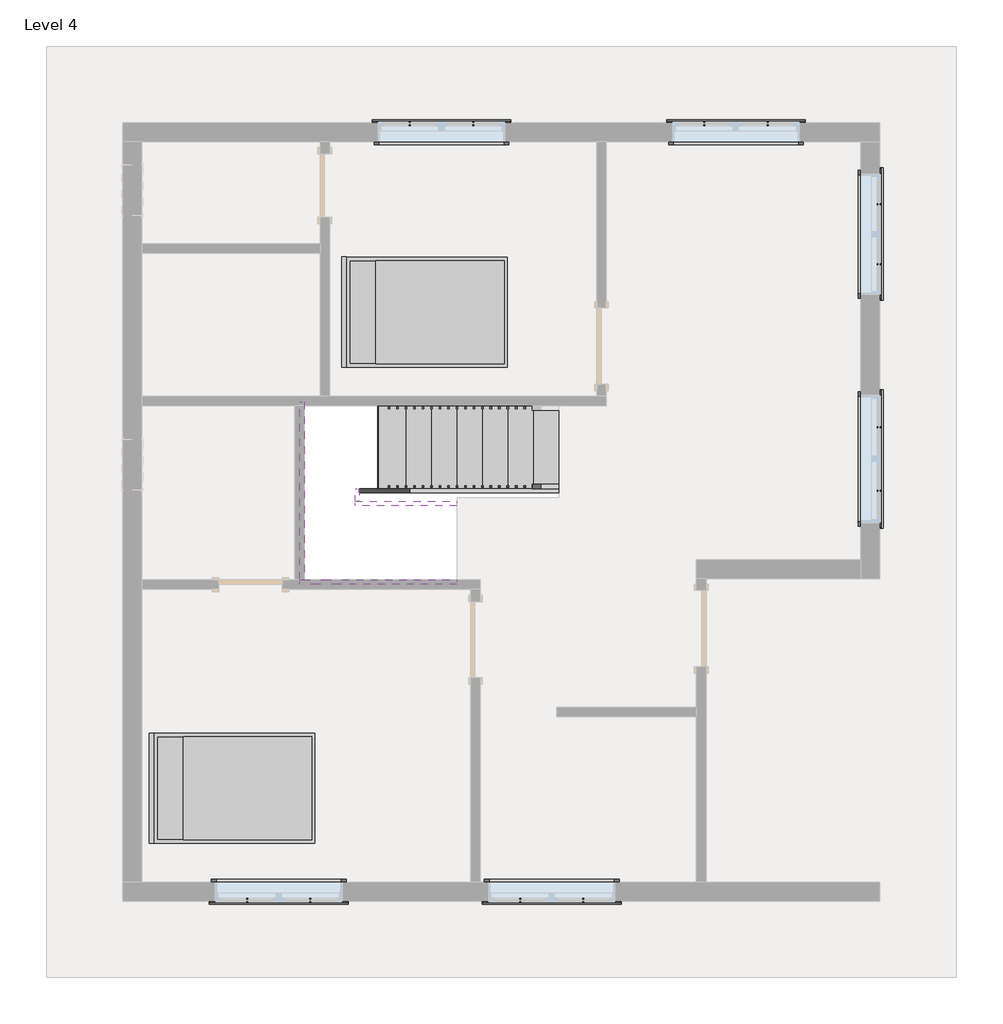
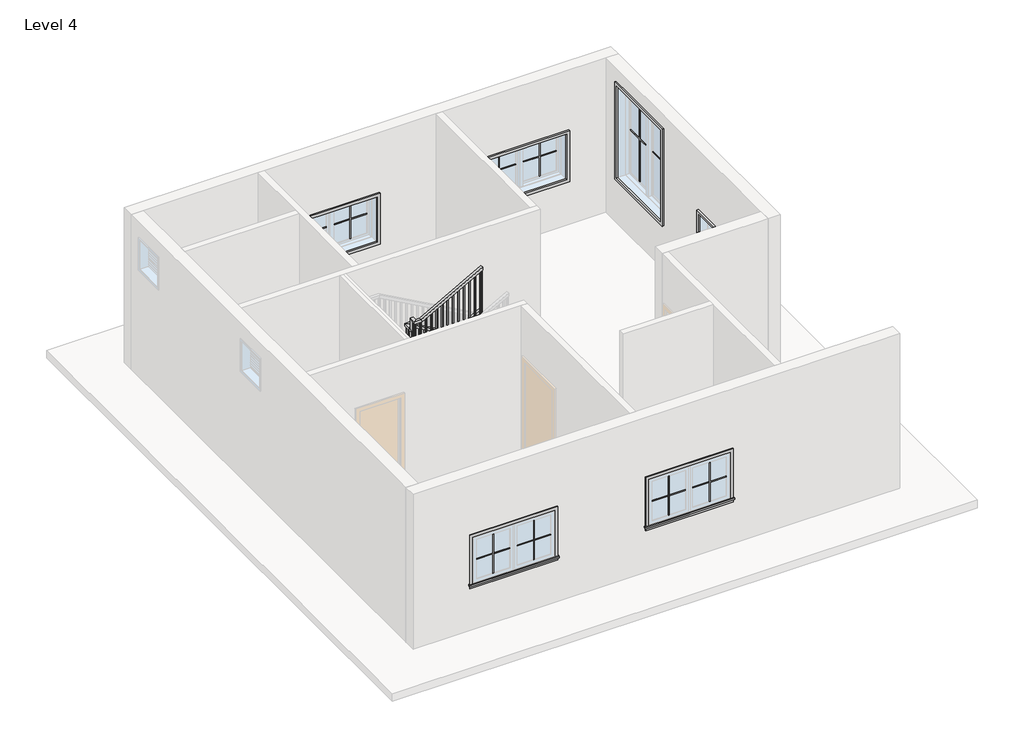
# One storey, part 2 of 2: 24 proxies, 6 members, 2 furniture elements, 1 railing, 1 stair flight.
"""IFC4 building model written with IfcOpenShell, lengths in millimetres."""

from ifc_helpers import new_model, si_unit, frame, origin, place, context, project, spatial, polyline, outline, extrude, faceted_brep, transform, mapped, element, save
from components import muntin_pattern_2x2_muntin_pattern_2x2_9352d081, muntin_pattern_2x2_muntin_pattern_2x2_5c2cbe28, muntin_pattern_2x2_muntin_pattern_2x2_bff912c5, muntin_pattern_2x2_muntin_pattern_2x2_c2194282, trim_window_exterior_flat_with_sill_979bde60, trim_window_exterior_flat_with_sill_e04b3088, trim_window_interior_flat_picture_frame_7883d11b, trim_window_interior_flat_picture_frame_2a7685fe, bed_17739_bed_17739_15c61121, stair_flight_db34188c

model = new_model("IFC4")

# Units and contexts
model_context = context("Model", 3, world=origin())
ifc_project = project(units=[si_unit("LENGTHUNIT", "METRE", prefix="MILLI")], contexts=[model_context])

# Site, building, storey
site = spatial("IfcSite", under=ifc_project)
building = spatial("IfcBuilding", under=site)
storey = spatial("IfcBuildingStorey", under=building, Name="Level 4", Elevation=9448.8)

# Proxies
placement = place(None, origin())
muntin_pattern_2x2_muntin_pattern_2x2_shape = muntin_pattern_2x2_muntin_pattern_2x2_9352d081(model_context)
element("IfcBuildingElementProxy", 1, Name="Muntin Pattern_2x2 : Muntin Pattern_2x2", ObjectType="Muntin Pattern_2x2 : Muntin Pattern_2x2", at=placement, inside=storey, context=model_context, shape_type="MappedRepresentation", body=[
    mapped(muntin_pattern_2x2_muntin_pattern_2x2_shape, transform((-3542.9505704, -5264.0292021, 10433.05), x_axis=(-1.0, 0.0, 0.0), y_axis=(0.0, -1.0, 0.0), z_axis=(0.0, 0.0, 1.0))),
])
element("IfcBuildingElementProxy", 2, Name="Muntin Pattern_2x2 : Muntin Pattern_2x2", ObjectType="Muntin Pattern_2x2 : Muntin Pattern_2x2", at=placement, inside=storey, context=model_context, shape_type="MappedRepresentation", body=[
    mapped(muntin_pattern_2x2_muntin_pattern_2x2_shape, transform((-272.7005704, -5264.0292021, 10433.05), x_axis=(-1.0, 0.0, 0.0), y_axis=(0.0, -1.0, 0.0), z_axis=(0.0, 0.0, 1.0))),
])
element("IfcBuildingElementProxy", 3, Name="Muntin Pattern_2x2 : Muntin Pattern_2x2", ObjectType="Muntin Pattern_2x2 : Muntin Pattern_2x2", at=placement, inside=storey, context=model_context, shape_type="MappedRepresentation", body=[
    mapped(muntin_pattern_2x2_muntin_pattern_2x2_shape, transform((3269.0119296, 401.7582979, 10433.05), x_axis=(0.0, -1.0, 0.0), y_axis=(1.0, 0.0, 0.0), z_axis=(0.0, 0.0, 1.0))),
])
element("IfcBuildingElementProxy", 4, Name="Muntin Pattern_2x2 : Muntin Pattern_2x2", ObjectType="Muntin Pattern_2x2 : Muntin Pattern_2x2", at=placement, inside=storey, context=model_context, shape_type="MappedRepresentation", body=[
    mapped(muntin_pattern_2x2_muntin_pattern_2x2_shape, transform((1175.0994296, 4038.7207979, 10433.05), x_axis=(1.0, 0.0, 0.0), y_axis=(0.0, 1.0, 0.0), z_axis=(0.0, 0.0, 1.0))),
])
element("IfcBuildingElementProxy", 5, Name="Muntin Pattern_2x2 : Muntin Pattern_2x2", ObjectType="Muntin Pattern_2x2 : Muntin Pattern_2x2", at=placement, inside=storey, context=model_context, shape_type="MappedRepresentation", body=[
    mapped(muntin_pattern_2x2_muntin_pattern_2x2_shape, transform((-2352.3255704, 4038.7207979, 10433.05), x_axis=(1.0, 0.0, 0.0), y_axis=(0.0, 1.0, 0.0), z_axis=(0.0, 0.0, 1.0))),
])
muntin_pattern_2x2_muntin_pattern_2x2_2_shape = muntin_pattern_2x2_muntin_pattern_2x2_5c2cbe28(model_context)
element("IfcBuildingElementProxy", 6, Name="Muntin Pattern_2x2 : Muntin Pattern_2x2", ObjectType="Muntin Pattern_2x2 : Muntin Pattern_2x2", at=placement, inside=storey, context=model_context, shape_type="MappedRepresentation", body=[
    mapped(muntin_pattern_2x2_muntin_pattern_2x2_2_shape, transform((-4301.7755704, -5264.0292021, 10433.05), x_axis=(1.0, 0.0, 0.0), y_axis=(0.0, 1.0, 0.0), z_axis=(0.0, 0.0, 1.0))),
])
element("IfcBuildingElementProxy", 7, Name="Muntin Pattern_2x2 : Muntin Pattern_2x2", ObjectType="Muntin Pattern_2x2 : Muntin Pattern_2x2", at=placement, inside=storey, context=model_context, shape_type="MappedRepresentation", body=[
    mapped(muntin_pattern_2x2_muntin_pattern_2x2_2_shape, transform((-1031.5255704, -5264.0292021, 10433.05), x_axis=(1.0, 0.0, 0.0), y_axis=(0.0, 1.0, 0.0), z_axis=(0.0, 0.0, 1.0))),
])
element("IfcBuildingElementProxy", 8, Name="Muntin Pattern_2x2 : Muntin Pattern_2x2", ObjectType="Muntin Pattern_2x2 : Muntin Pattern_2x2", at=placement, inside=storey, context=model_context, shape_type="MappedRepresentation", body=[
    mapped(muntin_pattern_2x2_muntin_pattern_2x2_2_shape, transform((3269.0119296, -357.0667021, 10433.05), x_axis=(0.0, 1.0, 0.0), y_axis=(-1.0, 0.0, 0.0), z_axis=(0.0, 0.0, 1.0))),
])
element("IfcBuildingElementProxy", 9, Name="Muntin Pattern_2x2 : Muntin Pattern_2x2", ObjectType="Muntin Pattern_2x2 : Muntin Pattern_2x2", at=placement, inside=storey, context=model_context, shape_type="MappedRepresentation", body=[
    mapped(muntin_pattern_2x2_muntin_pattern_2x2_2_shape, transform((1933.9244296, 4038.7207979, 10433.05), x_axis=(-1.0, 0.0, 0.0), y_axis=(0.0, -1.0, 0.0), z_axis=(0.0, 0.0, 1.0))),
])
element("IfcBuildingElementProxy", 10, Name="Muntin Pattern_2x2 : Muntin Pattern_2x2", ObjectType="Muntin Pattern_2x2 : Muntin Pattern_2x2", at=placement, inside=storey, context=model_context, shape_type="MappedRepresentation", body=[
    mapped(muntin_pattern_2x2_muntin_pattern_2x2_2_shape, transform((-1593.5005704, 4038.7207979, 10433.05), x_axis=(-1.0, 0.0, 0.0), y_axis=(0.0, -1.0, 0.0), z_axis=(0.0, 0.0, 1.0))),
])
muntin_pattern_2x2_muntin_pattern_2x2_3_shape = muntin_pattern_2x2_muntin_pattern_2x2_bff912c5(model_context)
element("IfcBuildingElementProxy", 11, Name="Muntin Pattern_2x2 : Muntin Pattern_2x2", ObjectType="Muntin Pattern_2x2 : Muntin Pattern_2x2", at=placement, inside=storey, context=model_context, shape_type="MappedRepresentation", body=[
    mapped(muntin_pattern_2x2_muntin_pattern_2x2_3_shape, transform((3269.0119296, 3075.1082979, 10433.05), x_axis=(0.0, -1.0, 0.0), y_axis=(1.0, 0.0, 0.0), z_axis=(0.0, 0.0, 1.0))),
])
muntin_pattern_2x2_muntin_pattern_2x2_4_shape = muntin_pattern_2x2_muntin_pattern_2x2_c2194282(model_context)
element("IfcBuildingElementProxy", 12, Name="Muntin Pattern_2x2 : Muntin Pattern_2x2", ObjectType="Muntin Pattern_2x2 : Muntin Pattern_2x2", at=placement, inside=storey, context=model_context, shape_type="MappedRepresentation", body=[
    mapped(muntin_pattern_2x2_muntin_pattern_2x2_4_shape, transform((3269.0119296, 2354.3832979, 10433.05), x_axis=(0.0, 1.0, 0.0), y_axis=(-1.0, 0.0, 0.0), z_axis=(0.0, 0.0, 1.0))),
])
trim_window_exterior_flat_with_sill_shape = trim_window_exterior_flat_with_sill_979bde60(model_context)
element("IfcBuildingElementProxy", 13, Name="Trim-Window-Exterior-Flat : with Sill", ObjectType="Trim-Window-Exterior-Flat : with Sill", at=placement, inside=storey, context=model_context, shape_type="MappedRepresentation", body=[
    mapped(trim_window_exterior_flat_with_sill_shape, transform((-3922.3630704, -5273.5542021, 11277.6), x_axis=(1.0, 0.0, 0.0), y_axis=(0.0, 0.0, 1.0), z_axis=(0.0, -1.0, 0.0))),
])
element("IfcBuildingElementProxy", 14, Name="Trim-Window-Exterior-Flat : with Sill", ObjectType="Trim-Window-Exterior-Flat : with Sill", at=placement, inside=storey, context=model_context, shape_type="MappedRepresentation", body=[
    mapped(trim_window_exterior_flat_with_sill_shape, transform((-652.1130704, -5273.5542021, 11277.6), x_axis=(1.0, 0.0, 0.0), y_axis=(0.0, 0.0, 1.0), z_axis=(0.0, -1.0, 0.0))),
])
element("IfcBuildingElementProxy", 15, Name="Trim-Window-Exterior-Flat : with Sill", ObjectType="Trim-Window-Exterior-Flat : with Sill", at=placement, inside=storey, context=model_context, shape_type="MappedRepresentation", body=[
    mapped(trim_window_exterior_flat_with_sill_shape, transform((3278.5369296, 22.3457979, 11277.6), x_axis=(0.0, 1.0, 0.0), y_axis=(0.0, 0.0, 1.0), z_axis=(1.0, 0.0, 0.0))),
])
element("IfcBuildingElementProxy", 16, Name="Trim-Window-Exterior-Flat : with Sill", ObjectType="Trim-Window-Exterior-Flat : with Sill", at=placement, inside=storey, context=model_context, shape_type="MappedRepresentation", body=[
    mapped(trim_window_exterior_flat_with_sill_shape, transform((1554.5119296, 4048.2457979, 11277.6), x_axis=(-1.0, 0.0, 0.0), y_axis=(0.0, 0.0, 1.0), z_axis=(0.0, 1.0, 0.0))),
])
element("IfcBuildingElementProxy", 17, Name="Trim-Window-Exterior-Flat : with Sill", ObjectType="Trim-Window-Exterior-Flat : with Sill", at=placement, inside=storey, context=model_context, shape_type="MappedRepresentation", body=[
    mapped(trim_window_exterior_flat_with_sill_shape, transform((-1972.9130704, 4048.2457979, 11277.6), x_axis=(-1.0, 0.0, 0.0), y_axis=(0.0, 0.0, 1.0), z_axis=(0.0, 1.0, 0.0))),
])
trim_window_exterior_flat_with_sill_2_shape = trim_window_exterior_flat_with_sill_e04b3088(model_context)
element("IfcBuildingElementProxy", 18, Name="Trim-Window-Exterior-Flat : with Sill", ObjectType="Trim-Window-Exterior-Flat : with Sill", at=placement, inside=storey, context=model_context, shape_type="MappedRepresentation", body=[
    mapped(trim_window_exterior_flat_with_sill_2_shape, transform((3278.5369296, 2714.7457979, 12192.0), x_axis=(0.0, 1.0, 0.0), y_axis=(0.0, 0.0, 1.0), z_axis=(1.0, 0.0, 0.0))),
])
trim_window_interior_flat_picture_frame_shape = trim_window_interior_flat_picture_frame_7883d11b(model_context)
element("IfcBuildingElementProxy", 19, Name="Trim-Window-Interior-Flat : Picture Frame", ObjectType="Trim-Window-Interior-Flat : Picture Frame", at=placement, inside=storey, context=model_context, shape_type="MappedRepresentation", body=[
    mapped(trim_window_interior_flat_picture_frame_shape, transform((-3922.3630704, -5044.9542021, 11277.6), x_axis=(-1.0, 0.0, 0.0), y_axis=(0.0, 0.0, 1.0), z_axis=(0.0, 1.0, 0.0))),
])
element("IfcBuildingElementProxy", 20, Name="Trim-Window-Interior-Flat : Picture Frame", ObjectType="Trim-Window-Interior-Flat : Picture Frame", at=placement, inside=storey, context=model_context, shape_type="MappedRepresentation", body=[
    mapped(trim_window_interior_flat_picture_frame_shape, transform((-652.1130704, -5044.9542021, 11277.6), x_axis=(-1.0, 0.0, 0.0), y_axis=(0.0, 0.0, 1.0), z_axis=(0.0, 1.0, 0.0))),
])
element("IfcBuildingElementProxy", 21, Name="Trim-Window-Interior-Flat : Picture Frame", ObjectType="Trim-Window-Interior-Flat : Picture Frame", at=placement, inside=storey, context=model_context, shape_type="MappedRepresentation", body=[
    mapped(trim_window_interior_flat_picture_frame_shape, transform((3049.9369296, 22.3457979, 11277.6), x_axis=(0.0, -1.0, 0.0), y_axis=(0.0, 0.0, 1.0), z_axis=(-1.0, 0.0, 0.0))),
])
element("IfcBuildingElementProxy", 22, Name="Trim-Window-Interior-Flat : Picture Frame", ObjectType="Trim-Window-Interior-Flat : Picture Frame", at=placement, inside=storey, context=model_context, shape_type="MappedRepresentation", body=[
    mapped(trim_window_interior_flat_picture_frame_shape, transform((1554.5119296, 3819.6457979, 11277.6), x_axis=(1.0, 0.0, 0.0), y_axis=(0.0, 0.0, 1.0), z_axis=(0.0, -1.0, 0.0))),
])
element("IfcBuildingElementProxy", 23, Name="Trim-Window-Interior-Flat : Picture Frame", ObjectType="Trim-Window-Interior-Flat : Picture Frame", at=placement, inside=storey, context=model_context, shape_type="MappedRepresentation", body=[
    mapped(trim_window_interior_flat_picture_frame_shape, transform((-1972.9130704, 3819.6457979, 11277.6), x_axis=(1.0, 0.0, 0.0), y_axis=(0.0, 0.0, 1.0), z_axis=(0.0, -1.0, 0.0))),
])
trim_window_interior_flat_picture_frame_2_shape = trim_window_interior_flat_picture_frame_2a7685fe(model_context)
element("IfcBuildingElementProxy", 24, Name="Trim-Window-Interior-Flat : Picture Frame", ObjectType="Trim-Window-Interior-Flat : Picture Frame", at=placement, inside=storey, context=model_context, shape_type="MappedRepresentation", body=[
    mapped(trim_window_interior_flat_picture_frame_2_shape, transform((3049.9369296, 2714.7457979, 12192.0), x_axis=(0.0, -1.0, 0.0), y_axis=(0.0, 0.0, 1.0), z_axis=(-1.0, 0.0, 0.0))),
])

# Furniture
bed_17739_bed_17739_shape = bed_17739_bed_17739_15c61121(model_context)
element("IfcFurniture", 25, ObjectType="Bed_17739 : Bed_17739", at=placement, inside=storey, context=model_context, shape_type="MappedRepresentation", body=[
    mapped(bed_17739_bed_17739_shape, transform((-4455.7630704, -3920.5467683, 9448.8), x_axis=(0.0, 1.0, 0.0), y_axis=(-1.0, 0.0, 0.0), z_axis=(0.0, 0.0, 1.0))),
])
element("IfcFurniture", 26, ObjectType="Bed_17739 : Bed_17739", at=placement, inside=storey, context=model_context, shape_type="MappedRepresentation", body=[
    mapped(bed_17739_bed_17739_shape, transform((-2150.7130704, 1781.2957979, 9448.8), x_axis=(0.0, 1.0, 0.0), y_axis=(-1.0, 0.0, 0.0), z_axis=(0.0, 0.0, 1.0))),
])

# Members
element("IfcMember", 27, ObjectType="Stringer - 2\" Width", at=placement, inside=storey, context=model_context, shape_type="SweptSolid", body=[
    extrude(outline(polyline([(9448.8, -569.5630704), (9656.3983948, -569.5630704), (10982.8428392, -2957.1630704), (10634.1641651, -2957.1630704), (9448.8, -823.5075732), (9448.8, -569.5630704)])), frame((0.0, -384.0542021, 0.0), z_axis=(0.0, 1.0, 0.0), x_axis=(0.0, 0.0, 1.0)), (0.0, 0.0, 1.0), 50.8),
])
element("IfcMember", 28, ObjectType="Stringer - 2\" Width", at=placement, inside=storey, context=model_context, shape_type="SweptSolid", body=[
    extrude(outline(polyline([(-3007.9630704, -333.2542021), (-2957.1630704, -333.2542021), (-2957.1630704, -485.6542021), (-3007.9630704, -485.6542021), (-3007.9630704, -333.2542021)])), frame((0.0, 0.0, 10744.2), z_axis=(0.0, 0.0, 1.0), x_axis=(1.0, 0.0, 0.0)), (0.0, 0.0, 1.0), 304.8),
])
element("IfcMember", 29, ObjectType="Stringer - 2\" Width", at=placement, inside=storey, context=model_context, shape_type="SweptSolid", body=[
    extrude(outline(polyline([(11180.3983948, -3007.9630704), (10831.7197207, -3007.9630704), (11509.053054, -1788.7630704), (11857.7317281, -1788.7630704), (11180.3983948, -3007.9630704)])), frame((0.0, -536.4542021, 0.0), z_axis=(0.0, 1.0, 0.0), x_axis=(0.0, 0.0, 1.0)), (0.0, 0.0, 1.0), 50.8),
])
element("IfcMember", 30, ObjectType="Stringer - 2\" Width", at=placement, inside=storey, context=model_context, shape_type="SweptSolid", body=[
    extrude(outline(polyline([(9448.8, -569.5630704), (9656.3983948, -569.5630704), (11049.0, -3076.2459598), (11049.0, -3617.5630704), (11001.053054, -3617.5630704), (9448.8, -823.5075732), (9448.8, -569.5630704)])), frame((0.0, 657.3457979, 0.0), z_axis=(0.0, 1.0, 0.0), x_axis=(0.0, 0.0, 1.0)), (0.0, 0.0, 1.0), 50.8),
])
element("IfcMember", 31, ObjectType="Stringer - 2\" Width", at=placement, inside=storey, context=model_context, shape_type="SweptSolid", body=[
    extrude(outline(polyline([(-3668.3630704, 708.1457979), (-3617.5630704, 708.1457979), (-3617.5630704, -1425.4542021), (-3668.3630704, -1425.4542021), (-3668.3630704, 708.1457979)])), frame((0.0, 0.0, 10744.2), z_axis=(0.0, 0.0, 1.0), x_axis=(1.0, 0.0, 0.0)), (0.0, 0.0, 1.0), 304.8),
])
element("IfcMember", 32, ObjectType="Stringer - 2\" Width", at=placement, inside=storey, context=model_context, shape_type="SweptSolid", body=[
    extrude(outline(polyline([(10813.5095059, -3668.3630704), (10744.2, -3668.3630704), (10744.2, -3165.4985677), (11509.053054, -1788.7630704), (11857.7317281, -1788.7630704), (10813.5095059, -3668.3630704)])), frame((0.0, -1476.2542021, 0.0), z_axis=(0.0, 1.0, 0.0), x_axis=(0.0, 0.0, 1.0)), (0.0, 0.0, 1.0), 50.8),
])

# Railing
element("IfcRailing", 33, ObjectType="Handrail - Rectangular", at=placement, inside=storey, context=model_context, shape_type="SolidModel", body=[
    faceted_brep([(-569.5630704, -333.2542021, 10532.5333333), (-569.5630704, -333.2542021, 10474.420221), (-569.5630704, -282.4542021, 10474.420221), (-569.5630704, -282.4542021, 10532.5333333), (-2931.7630704, -333.2542021, 11844.8666667), (-2982.5630704, -333.2542021, 11814.9757765), (-2982.5630704, -282.4542021, 11814.9757765), (-2931.7630704, -282.4542021, 11844.8666667), (-2931.7630704, -333.2542021, 11887.2), (-2982.5630704, -333.2542021, 11836.4), (-2982.5630704, -282.4542021, 11836.4), (-2931.7630704, -282.4542021, 11887.2), (-3007.9630704, -333.2542021, 11887.2), (-3007.9630704, -333.2542021, 11836.4), (-3058.7630704, -282.4542021, 11836.4), (-3058.7630704, -282.4542021, 11887.2), (-3007.9630704, -409.4542021, 11887.2), (-3007.9630704, -409.4542021, 11836.4), (-3058.7630704, -409.4542021, 11836.4), (-3058.7630704, -409.4542021, 11887.2), (-3007.9630704, -460.2542021, 11887.2), (-3007.9630704, -511.0542021, 11836.4), (-3058.7630704, -511.0542021, 11836.4), (-3058.7630704, -460.2542021, 11887.2), (-3007.9630704, -460.2542021, 12098.8666667), (-3007.9630704, -511.0542021, 12048.0666667), (-3058.7630704, -511.0542021, 12048.0666667), (-3058.7630704, -460.2542021, 12098.8666667), (-3007.9630704, -536.4542021, 12098.8666667), (-3007.9630704, -536.4542021, 12048.0666667), (-3058.7630704, -587.2542021, 12048.0666667), (-3058.7630704, -587.2542021, 12098.8666667), (-2931.7630704, -536.4542021, 12098.8666667), (-2918.5994682, -536.4542021, 12048.0666667), (-2918.5994682, -587.2542021, 12048.0666667), (-2931.7630704, -587.2542021, 12098.8666667), (-1788.7630704, -536.4542021, 12733.8666667), (-1788.7630704, -587.2542021, 12733.8666667), (-1788.7630704, -587.2542021, 12675.7535543), (-1788.7630704, -536.4542021, 12675.7535543)], [[[0, 1, 2, 3]], [[1, 0, 4, 5]], [[2, 1, 5, 6]], [[3, 2, 6, 7]], [[0, 3, 7, 4]], [[5, 4, 8, 9]], [[6, 5, 9, 10]], [[7, 6, 10, 11]], [[4, 7, 11, 8]], [[9, 8, 12, 13]], [[10, 9, 13, 14]], [[11, 10, 14, 15]], [[8, 11, 15, 12]], [[13, 12, 16, 17]], [[14, 13, 17, 18]], [[15, 14, 18, 19]], [[12, 15, 19, 16]], [[17, 16, 20, 21]], [[18, 17, 21, 22]], [[19, 18, 22, 23]], [[16, 19, 23, 20]], [[21, 20, 24, 25]], [[22, 21, 25, 26]], [[23, 22, 26, 27]], [[20, 23, 27, 24]], [[25, 24, 28, 29]], [[26, 25, 29, 30]], [[27, 26, 30, 31]], [[24, 27, 31, 28]], [[29, 28, 32, 33]], [[30, 29, 33, 34]], [[31, 30, 34, 35]], [[28, 31, 35, 32]], [[36, 37, 38, 39]], [[33, 32, 36, 39]], [[34, 33, 39, 38]], [[35, 34, 38, 37]], [[32, 35, 37, 36]]]),
    extrude(outline(polyline([(12656.3507765, -1823.6880704), (11650.1333333, -1823.6880704), (11650.1333333, -1804.6380704), (12666.9341099, -1804.6380704), (12656.3507765, -1823.6880704)])), frame((0.0, -571.3792021, 0.0), z_axis=(0.0, 1.0, 0.0), x_axis=(0.0, 0.0, 1.0)), (0.0, 0.0, 1.0), 19.05),
    extrude(outline(polyline([(12599.9063321, -1925.2880704), (11650.1333333, -1925.2880704), (11650.1333333, -1906.2380704), (12610.4896654, -1906.2380704), (12599.9063321, -1925.2880704)])), frame((0.0, -571.3792021, 0.0), z_axis=(0.0, 1.0, 0.0), x_axis=(0.0, 0.0, 1.0)), (0.0, 0.0, 1.0), 19.05),
    extrude(outline(polyline([(12543.4618876, -2026.8880704), (11650.1333333, -2026.8880704), (11650.1333333, -2007.8380704), (12554.045221, -2007.8380704), (12543.4618876, -2026.8880704)])), frame((0.0, -571.3792021, 0.0), z_axis=(0.0, 1.0, 0.0), x_axis=(0.0, 0.0, 1.0)), (0.0, 0.0, 1.0), 19.05),
    extrude(outline(polyline([(12487.0174432, -2128.4880704), (11480.8, -2128.4880704), (11480.8, -2109.4380704), (12497.6007765, -2109.4380704), (12487.0174432, -2128.4880704)])), frame((0.0, -571.3792021, 0.0), z_axis=(0.0, 1.0, 0.0), x_axis=(0.0, 0.0, 1.0)), (0.0, 0.0, 1.0), 19.05),
    extrude(outline(polyline([(12430.5729988, -2230.0880704), (11480.8, -2230.0880704), (11480.8, -2211.0380704), (12441.1563321, -2211.0380704), (12430.5729988, -2230.0880704)])), frame((0.0, -571.3792021, 0.0), z_axis=(0.0, 1.0, 0.0), x_axis=(0.0, 0.0, 1.0)), (0.0, 0.0, 1.0), 19.05),
    extrude(outline(polyline([(12374.1285543, -2331.6880704), (11480.8, -2331.6880704), (11480.8, -2312.6380704), (12384.7118876, -2312.6380704), (12374.1285543, -2331.6880704)])), frame((0.0, -571.3792021, 0.0), z_axis=(0.0, 1.0, 0.0), x_axis=(0.0, 0.0, 1.0)), (0.0, 0.0, 1.0), 19.05),
    extrude(outline(polyline([(12317.6841099, -2433.2880704), (11311.4666667, -2433.2880704), (11311.4666667, -2414.2380704), (12328.2674432, -2414.2380704), (12317.6841099, -2433.2880704)])), frame((0.0, -571.3792021, 0.0), z_axis=(0.0, 1.0, 0.0), x_axis=(0.0, 0.0, 1.0)), (0.0, 0.0, 1.0), 19.05),
    extrude(outline(polyline([(12261.2396654, -2534.8880704), (11311.4666667, -2534.8880704), (11311.4666667, -2515.8380704), (12271.8229988, -2515.8380704), (12261.2396654, -2534.8880704)])), frame((0.0, -571.3792021, 0.0), z_axis=(0.0, 1.0, 0.0), x_axis=(0.0, 0.0, 1.0)), (0.0, 0.0, 1.0), 19.05),
    extrude(outline(polyline([(12204.795221, -2636.4880704), (11311.4666667, -2636.4880704), (11311.4666667, -2617.4380704), (12215.3785543, -2617.4380704), (12204.795221, -2636.4880704)])), frame((0.0, -571.3792021, 0.0), z_axis=(0.0, 1.0, 0.0), x_axis=(0.0, 0.0, 1.0)), (0.0, 0.0, 1.0), 19.05),
    extrude(outline(polyline([(12148.3507765, -2738.0880704), (11142.1333333, -2738.0880704), (11142.1333333, -2719.0380704), (12158.9341099, -2719.0380704), (12148.3507765, -2738.0880704)])), frame((0.0, -571.3792021, 0.0), z_axis=(0.0, 1.0, 0.0), x_axis=(0.0, 0.0, 1.0)), (0.0, 0.0, 1.0), 19.05),
    extrude(outline(polyline([(12091.9063321, -2839.6880704), (11142.1333333, -2839.6880704), (11142.1333333, -2820.6380704), (12102.4896654, -2820.6380704), (12091.9063321, -2839.6880704)])), frame((0.0, -571.3792021, 0.0), z_axis=(0.0, 1.0, 0.0), x_axis=(0.0, 0.0, 1.0)), (0.0, 0.0, 1.0), 19.05),
    extrude(outline(polyline([(12035.4618876, -2941.2880704), (11142.1333333, -2941.2880704), (11142.1333333, -2922.2380704), (12046.045221, -2922.2380704), (12035.4618876, -2941.2880704)])), frame((0.0, -571.3792021, 0.0), z_axis=(0.0, 1.0, 0.0), x_axis=(0.0, 0.0, 1.0)), (0.0, 0.0, 1.0), 19.05),
    extrude(outline(polyline([(-3023.8380704, -501.5292021), (-3023.8380704, -520.5792021), (-3042.8880704, -520.5792021), (-3042.8880704, -501.5292021), (-3023.8380704, -501.5292021)])), frame((0.0, 0.0, 10972.8), z_axis=(0.0, 0.0, 1.0), x_axis=(1.0, 0.0, 0.0)), (0.0, 0.0, 1.0), 1075.2666667),
    extrude(outline(polyline([(-3023.8380704, -399.9292021), (-3023.8380704, -418.9792021), (-3042.8880704, -418.9792021), (-3042.8880704, -399.9292021), (-3023.8380704, -399.9292021)])), frame((0.0, 0.0, 10972.8), z_axis=(0.0, 0.0, 1.0), x_axis=(1.0, 0.0, 0.0)), (0.0, 0.0, 1.0), 863.6),
    extrude(outline(polyline([(-2998.4380704, -317.3792021), (-3017.4880704, -317.3792021), (-3017.4880704, -298.3292021), (-2998.4380704, -298.3292021), (-2998.4380704, -317.3792021)])), frame((0.0, 0.0, 10972.8), z_axis=(0.0, 0.0, 1.0), x_axis=(1.0, 0.0, 0.0)), (0.0, 0.0, 1.0), 863.6),
    extrude(outline(polyline([(11777.9341099, -2915.8880704), (10803.4666667, -2915.8880704), (10803.4666667, -2896.8380704), (11767.3507765, -2896.8380704), (11777.9341099, -2915.8880704)])), frame((0.0, -317.3792021, 0.0), z_axis=(0.0, 1.0, 0.0), x_axis=(0.0, 0.0, 1.0)), (0.0, 0.0, 1.0), 19.05),
    extrude(outline(polyline([(11721.4896654, -2814.2880704), (10803.4666667, -2814.2880704), (10803.4666667, -2795.2380704), (11710.9063321, -2795.2380704), (11721.4896654, -2814.2880704)])), frame((0.0, -317.3792021, 0.0), z_axis=(0.0, 1.0, 0.0), x_axis=(0.0, 0.0, 1.0)), (0.0, 0.0, 1.0), 19.05),
    extrude(outline(polyline([(11665.045221, -2712.6880704), (10803.4666667, -2712.6880704), (10803.4666667, -2693.6380704), (11654.4618876, -2693.6380704), (11665.045221, -2712.6880704)])), frame((0.0, -317.3792021, 0.0), z_axis=(0.0, 1.0, 0.0), x_axis=(0.0, 0.0, 1.0)), (0.0, 0.0, 1.0), 19.05),
    extrude(outline(polyline([(11608.6007765, -2611.0880704), (10634.1333333, -2611.0880704), (10634.1333333, -2592.0380704), (11598.0174432, -2592.0380704), (11608.6007765, -2611.0880704)])), frame((0.0, -317.3792021, 0.0), z_axis=(0.0, 1.0, 0.0), x_axis=(0.0, 0.0, 1.0)), (0.0, 0.0, 1.0), 19.05),
    extrude(outline(polyline([(11552.1563321, -2509.4880704), (10634.1333333, -2509.4880704), (10634.1333333, -2490.4380704), (11541.5729988, -2490.4380704), (11552.1563321, -2509.4880704)])), frame((0.0, -317.3792021, 0.0), z_axis=(0.0, 1.0, 0.0), x_axis=(0.0, 0.0, 1.0)), (0.0, 0.0, 1.0), 19.05),
    extrude(outline(polyline([(11495.7118876, -2407.8880704), (10634.1333333, -2407.8880704), (10634.1333333, -2388.8380704), (11485.1285543, -2388.8380704), (11495.7118876, -2407.8880704)])), frame((0.0, -317.3792021, 0.0), z_axis=(0.0, 1.0, 0.0), x_axis=(0.0, 0.0, 1.0)), (0.0, 0.0, 1.0), 19.05),
    extrude(outline(polyline([(11439.2674432, -2306.2880704), (10464.8, -2306.2880704), (10464.8, -2287.2380704), (11428.6841099, -2287.2380704), (11439.2674432, -2306.2880704)])), frame((0.0, -317.3792021, 0.0), z_axis=(0.0, 1.0, 0.0), x_axis=(0.0, 0.0, 1.0)), (0.0, 0.0, 1.0), 19.05),
    extrude(outline(polyline([(11382.8229988, -2204.6880704), (10464.8, -2204.6880704), (10464.8, -2185.6380704), (11372.2396654, -2185.6380704), (11382.8229988, -2204.6880704)])), frame((0.0, -317.3792021, 0.0), z_axis=(0.0, 1.0, 0.0), x_axis=(0.0, 0.0, 1.0)), (0.0, 0.0, 1.0), 19.05),
    extrude(outline(polyline([(11326.3785543, -2103.0880704), (10464.8, -2103.0880704), (10464.8, -2084.0380704), (11315.795221, -2084.0380704), (11326.3785543, -2103.0880704)])), frame((0.0, -317.3792021, 0.0), z_axis=(0.0, 1.0, 0.0), x_axis=(0.0, 0.0, 1.0)), (0.0, 0.0, 1.0), 19.05),
    extrude(outline(polyline([(11269.9341099, -2001.4880704), (10295.4666667, -2001.4880704), (10295.4666667, -1982.4380704), (11259.3507765, -1982.4380704), (11269.9341099, -2001.4880704)])), frame((0.0, -317.3792021, 0.0), z_axis=(0.0, 1.0, 0.0), x_axis=(0.0, 0.0, 1.0)), (0.0, 0.0, 1.0), 19.05),
    extrude(outline(polyline([(11213.4896654, -1899.8880704), (10295.4666667, -1899.8880704), (10295.4666667, -1880.8380704), (11202.9063321, -1880.8380704), (11213.4896654, -1899.8880704)])), frame((0.0, -317.3792021, 0.0), z_axis=(0.0, 1.0, 0.0), x_axis=(0.0, 0.0, 1.0)), (0.0, 0.0, 1.0), 19.05),
    extrude(outline(polyline([(11157.045221, -1798.2880704), (10295.4666667, -1798.2880704), (10295.4666667, -1779.2380704), (11146.4618876, -1779.2380704), (11157.045221, -1798.2880704)])), frame((0.0, -317.3792021, 0.0), z_axis=(0.0, 1.0, 0.0), x_axis=(0.0, 0.0, 1.0)), (0.0, 0.0, 1.0), 19.05),
    extrude(outline(polyline([(11100.6007765, -1696.6880704), (10126.1333333, -1696.6880704), (10126.1333333, -1677.6380704), (11090.0174432, -1677.6380704), (11100.6007765, -1696.6880704)])), frame((0.0, -317.3792021, 0.0), z_axis=(0.0, 1.0, 0.0), x_axis=(0.0, 0.0, 1.0)), (0.0, 0.0, 1.0), 19.05),
    extrude(outline(polyline([(11044.1563321, -1595.0880704), (10126.1333333, -1595.0880704), (10126.1333333, -1576.0380704), (11033.5729988, -1576.0380704), (11044.1563321, -1595.0880704)])), frame((0.0, -317.3792021, 0.0), z_axis=(0.0, 1.0, 0.0), x_axis=(0.0, 0.0, 1.0)), (0.0, 0.0, 1.0), 19.05),
    extrude(outline(polyline([(10987.7118876, -1493.4880704), (10126.1333333, -1493.4880704), (10126.1333333, -1474.4380704), (10977.1285543, -1474.4380704), (10987.7118876, -1493.4880704)])), frame((0.0, -317.3792021, 0.0), z_axis=(0.0, 1.0, 0.0), x_axis=(0.0, 0.0, 1.0)), (0.0, 0.0, 1.0), 19.05),
    extrude(outline(polyline([(10931.2674432, -1391.8880704), (9956.8, -1391.8880704), (9956.8, -1372.8380704), (10920.6841099, -1372.8380704), (10931.2674432, -1391.8880704)])), frame((0.0, -317.3792021, 0.0), z_axis=(0.0, 1.0, 0.0), x_axis=(0.0, 0.0, 1.0)), (0.0, 0.0, 1.0), 19.05),
    extrude(outline(polyline([(10874.8229988, -1290.2880704), (9956.8, -1290.2880704), (9956.8, -1271.2380704), (10864.2396654, -1271.2380704), (10874.8229988, -1290.2880704)])), frame((0.0, -317.3792021, 0.0), z_axis=(0.0, 1.0, 0.0), x_axis=(0.0, 0.0, 1.0)), (0.0, 0.0, 1.0), 19.05),
    extrude(outline(polyline([(10818.3785543, -1188.6880704), (9956.8, -1188.6880704), (9956.8, -1169.6380704), (10807.795221, -1169.6380704), (10818.3785543, -1188.6880704)])), frame((0.0, -317.3792021, 0.0), z_axis=(0.0, 1.0, 0.0), x_axis=(0.0, 0.0, 1.0)), (0.0, 0.0, 1.0), 19.05),
    extrude(outline(polyline([(10761.9341099, -1087.0880704), (9787.4666667, -1087.0880704), (9787.4666667, -1068.0380704), (10751.3507765, -1068.0380704), (10761.9341099, -1087.0880704)])), frame((0.0, -317.3792021, 0.0), z_axis=(0.0, 1.0, 0.0), x_axis=(0.0, 0.0, 1.0)), (0.0, 0.0, 1.0), 19.05),
    extrude(outline(polyline([(10705.4896654, -985.4880704), (9787.4666667, -985.4880704), (9787.4666667, -966.4380704), (10694.9063321, -966.4380704), (10705.4896654, -985.4880704)])), frame((0.0, -317.3792021, 0.0), z_axis=(0.0, 1.0, 0.0), x_axis=(0.0, 0.0, 1.0)), (0.0, 0.0, 1.0), 19.05),
    extrude(outline(polyline([(10649.045221, -883.8880704), (9787.4666667, -883.8880704), (9787.4666667, -864.8380704), (10638.4618876, -864.8380704), (10649.045221, -883.8880704)])), frame((0.0, -317.3792021, 0.0), z_axis=(0.0, 1.0, 0.0), x_axis=(0.0, 0.0, 1.0)), (0.0, 0.0, 1.0), 19.05),
    extrude(outline(polyline([(10592.6007765, -782.2880704), (9618.1333333, -782.2880704), (9618.1333333, -763.2380704), (10582.0174432, -763.2380704), (10592.6007765, -782.2880704)])), frame((0.0, -317.3792021, 0.0), z_axis=(0.0, 1.0, 0.0), x_axis=(0.0, 0.0, 1.0)), (0.0, 0.0, 1.0), 19.05),
    extrude(outline(polyline([(10536.1563321, -680.6880704), (9618.1333333, -680.6880704), (9618.1333333, -661.6380704), (10525.5729988, -661.6380704), (10536.1563321, -680.6880704)])), frame((0.0, -317.3792021, 0.0), z_axis=(0.0, 1.0, 0.0), x_axis=(0.0, 0.0, 1.0)), (0.0, 0.0, 1.0), 19.05),
    extrude(outline(polyline([(-3023.8380704, -552.3292021), (-3023.8380704, -571.3792021), (-3042.8880704, -571.3792021), (-3042.8880704, -552.3292021), (-3023.8380704, -552.3292021)])), frame((0.0, 0.0, 10972.8), z_axis=(0.0, 0.0, 1.0), x_axis=(1.0, 0.0, 0.0)), (0.0, 0.0, 1.0), 1075.2666667),
    extrude(outline(polyline([(-3023.8380704, -317.3792021), (-3042.8880704, -317.3792021), (-3042.8880704, -298.3292021), (-3023.8380704, -298.3292021), (-3023.8380704, -317.3792021)])), frame((0.0, 0.0, 10972.8), z_axis=(0.0, 0.0, 1.0), x_axis=(1.0, 0.0, 0.0)), (0.0, 0.0, 1.0), 863.6),
    extrude(outline(polyline([(12665.170221, -1807.8130704), (11650.1333333, -1807.8130704), (11650.1333333, -1788.7630704), (12675.7535543, -1788.7630704), (12665.170221, -1807.8130704)])), frame((0.0, -571.3792021, 0.0), z_axis=(0.0, 1.0, 0.0), x_axis=(0.0, 0.0, 1.0)), (0.0, 0.0, 1.0), 19.05),
    extrude(outline(polyline([(10485.0035543, -588.6130704), (9618.1333333, -588.6130704), (9618.1333333, -569.5630704), (10474.420221, -569.5630704), (10485.0035543, -588.6130704)])), frame((0.0, -317.3792021, 0.0), z_axis=(0.0, 1.0, 0.0), x_axis=(0.0, 0.0, 1.0)), (0.0, 0.0, 1.0), 19.05),
])

# Stair flight
stair_flight_shape = stair_flight_db34188c(model_context)
element("IfcStairFlight", 34, ObjectType="2\" Tread 1\" Nosing 1/4\" Riser", at=placement, inside=storey, context=model_context, shape_type="MappedRepresentation", body=[
    mapped(stair_flight_shape, transform((0.0, 0.0, 0.0), x_axis=(1.0, 0.0, 0.0), y_axis=(0.0, 1.0, 0.0), z_axis=(0.0, 0.0, 1.0))),
])

save(model, "model.ifc")

# Revit data of these elements
# Type "Muntin Pattern_2x2 : Muntin Pattern_2x2"
#   Width [instance default] = 4' - 0"
#   Thickness = 0' - 0 1/2"
#   Height [instance default] = 4' - 0"
#   Distance = 0' - 0 3/4"
#   Interior Material [instance default] = none
#   Exterior Material [instance default] = none
#   Default Elevation = 0
# Type "Trim-Window-Exterior-Flat : with Sill"
#   Trim Width = 0' - 2 1/4"
#   Trim Thickness_Picture Frame = 0' - 1 1/4"
#   Trim Thickness_with Sill = 0' - 0 3/4"
#   Sill Thickness = 0' - 1 1/4"
#   Opening Width [instance default] = 2' - 0"
#   Opening Height [instance default] = 3' - 0"
#   Default Elevation = 4' - 0"
#   Sill = yes
#   Picture Frame = no
#   Trim Material [instance default] = none
# Type "Trim-Window-Interior-Flat : Picture Frame"
#   Trim Thickness_Picture Frame = 0' - 1 1/4"
#   Trim Width = 0' - 2 1/4"
#   Trim Thickness_with Sill = 0' - 0 3/4"
#   Sill Thickness = 0' - 1 1/4"
#   Opening Width [instance default] = 2' - 0"
#   Opening Height [instance default] = 3' - 0"
#   Default Elevation = 4' - 0"
#   Sill = no
#   Picture Frame = yes
#   Trim Material [instance default] = none
# Type "Bed_17739 : Bed_17739"
#   Default Elevation = 0
# Type "Handrail - Rectangular"
#   Assembly Code = "C2010400"
#   built-in parameter 1008612 = 0.0416667 (stored number, unit not read)
#   built-in parameter 1008611 = 0.0416667 (stored number, unit not read)
#   built-in parameter 1008609 = 0.333333 (stored number, unit not read)
#   built-in parameter 1008604 = 0.166667 (stored number, unit not read)
#   built-in parameter 1008603 = 0.166667 (stored number, unit not read)
#   Railing Height = 3' - 0"
#   built-in parameter 1008630 = 2
#   built-in parameter 1008610 = 2
#   built-in parameter 1008618 = Baluster - Square : 3/4"
# Elements 1, 2, 3, 4, 5, 6, 7, 8, 9, 10 (IfcBuildingElementProxy, "Muntin Pattern_2x2 : Muntin Pattern_2x2")
#   Width = 2' - 0 5/8"
#   Height = 2' - 6 1/2"
#   Interior Material = Wood - Stained
#   Exterior Material = Clad - White
#   Phase Created = New Construction
#   Materials on its faces: "Clad - White", "Wood - Stained"
# Elements 11, 12 (IfcBuildingElementProxy, "Muntin Pattern_2x2 : Muntin Pattern_2x2")
#   Width = 1' - 11 1/8"
#   Height = 5' - 6 1/2"
#   Interior Material = Wood - Stained
#   Exterior Material = Clad - White
#   Phase Created = New Construction
#   Materials on its faces: "Clad - White", "Wood - Stained"
# Elements 13, 14, 15, 16, 17 (IfcBuildingElementProxy, "Trim-Window-Exterior-Flat : with Sill")
#   Opening Width = 5' - 0"
#   Opening Height = 3' - 0"
#   Trim Material = Clad - White
#   Phase Created = New Construction
#   Materials on its faces: "Clad - White"
# Element 18 (IfcBuildingElementProxy, "Trim-Window-Exterior-Flat : with Sill")
#   Opening Width = 4' - 9"
#   Opening Height = 6' - 0"
#   Trim Material = Clad - White
#   Phase Created = New Construction
#   Materials on its faces: "Clad - White"
# Elements 19, 20, 21, 22, 23 (IfcBuildingElementProxy, "Trim-Window-Interior-Flat : Picture Frame")
#   Opening Width = 5' - 0"
#   Opening Height = 3' - 0"
#   Trim Material = Wood - Stained
#   Phase Created = New Construction
#   Materials on its faces: "Wood - Stained"
# Element 24 (IfcBuildingElementProxy, "Trim-Window-Interior-Flat : Picture Frame")
#   Opening Width = 4' - 9"
#   Opening Height = 6' - 0"
#   Trim Material = Wood - Stained
#   Phase Created = New Construction
#   Materials on its faces: "Wood - Stained"
# Elements 25, 26 (IfcFurniture, "Bed_17739 : Bed_17739")
#   Phase Created = New Construction
#   Materials on its faces: "legs", "sheets", "bed frame", "Blanket"
# Elements 27, 28, 29, 30, 31, 32 (IfcMember, "Stringer - 2\" Width")
#   Phase Created = New Construction
# Element 33 (IfcRailing, "Handrail - Rectangular")
#   Phase Created = New Construction
# Element 34 (IfcStairFlight, "2\" Tread 1\" Nosing 1/4\" Riser")
#   Phase Created = New Construction
# Materials
#   "Clad - White": class "Wood", colour RGB 242 242 238, transparency 0, Cost = 0
#   "Wood - Stained": class "Wood", colour RGB 224 178 126, transparency 0, Cost = 0
#   "legs": colour RGB 90 73 37, transparency 0, Cost = 0
#   "sheets": colour RGB 200 195 176, transparency 0, Cost = 0
#   "bed frame": colour RGB 90 73 37, transparency 0, Cost = 0
#   "Blanket": class "System", colour RGB 59 0 1, transparency 0, Cost = 0
